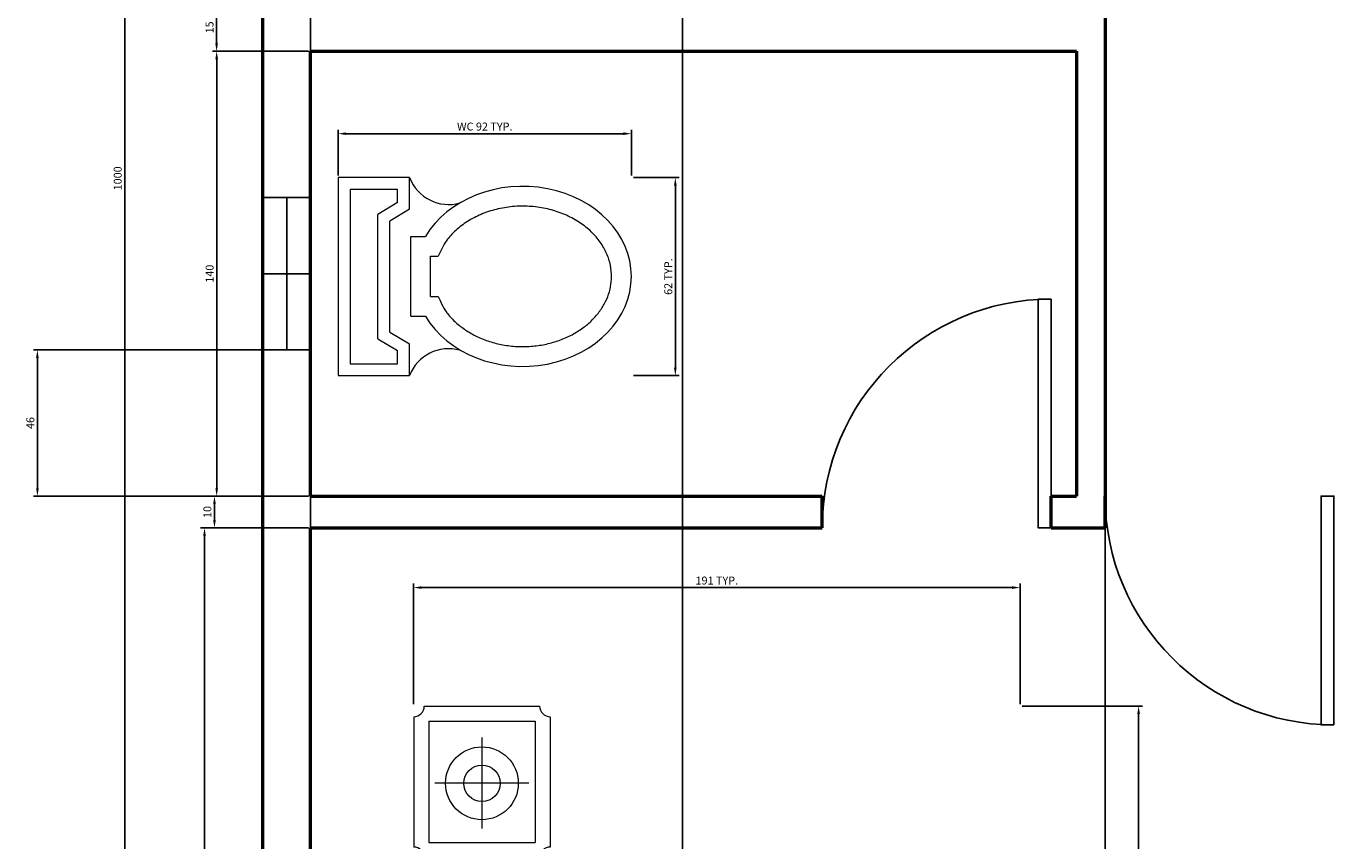
# Model space of a CAD drawing. Units: inches. Extents: x 604 to 3492, y -123 to 1737.
# Tile 12 of 20: x 1500 to 1912, y 579 to 836. Entities that reach past the tile are written whole.
import ezdxf

# ---------------------------------------------------------------- set-up
doc = ezdxf.new("R2010")
doc.units = ezdxf.units.IN
for name, color, linetype, lineweight in [('A-ANNO-DIMS', 2, 'Continuous', 18), ('A-DOOR', 3, 'Continuous', 25), ('A-FLOR-FIXT', 9, 'Continuous', 18), ('A-FURN', 8, 'Continuous', 18), ('A-GLAZ', 4, 'Continuous', 25), ('A-WALL', 7, 'Continuous', 50)]:
    doc.layers.add(name, color=color, linetype=linetype, lineweight=lineweight)
doc.styles.get("Standard").update_dxf_attribs({"font": 'arial.ttf'})
doc.dimstyles.new('ISO-25', dxfattribs={"dimtxt": 2.5, "dimasz": 2.5, "dimexe": 1.25, "dimexo": 0.625, "dimtad": 1, "dimtxsty": 'Standard', "dimcen": 2.5, "dimadec": 0, "dimazin": 0, "dimtfac": 1, "dimtmove": 0, "dimatfit": 3, "dimfxl": 1, "dimarcsym": 0})

# ---------------------------------------------------------------- blocks, each defined once
blk = doc.blocks.new('A$C7C8779AE')
for p, q in [((0, 0.7405), (0, 0.5605)), ((0.5, 0.7405), (0, 0.7405)), ((0.5, 0.5605), (0.5, 0.7405)), ((0.47, 0.7105), (0.03, 0.7105)), ((0.03, 0.7105), (0.03, 0.5905)), ((0.47, 0.5905), (0.47, 0.7105)), ((0.093, 0.6405), (0.063, 0.5905)), ((0.093, 0.6405), (0.407, 0.6405)), ((0.437, 0.5905), (0.407, 0.6405)), ((0.11, 0.6105), (0.08, 0.5605)), ((0.11, 0.6105), (0.39, 0.6105)), ((0.42, 0.5605), (0.39, 0.6105)), ((0.03, 0.5905), (0.063, 0.5905)), ((0.437, 0.5905), (0.47, 0.5905)), ((0, 0.5605), (0.08, 0.5605)), ((0.1497, 0.557), (0.1497, 0.5203)), ((0.1497, 0.557), (0.3514, 0.557)), ((0.3514, 0.557), (0.3514, 0.5203)), ((0.42, 0.5605), (0.5, 0.5605)), ((0.1997, 0.507), (0.1997, 0.4879)), ((0.1997, 0.507), (0.3014, 0.507)), ((0.3014, 0.507), (0.3014, 0.4879))]:
    blk.add_line(p, q)
for centre, start, end in [((-0.0386, 0.4613), 344.642, 68.7339), ((0.5386, 0.4613), 111.2661, 195.358)]:
    blk.add_arc(centre, 0.1064, start, end)
blk.add_ellipse((0.2506, 0.2744), major_axis=(0, 0.2744), ratio=0.828948, start_param=0.459479, end_param=5.823706)
blk.add_open_spline([(0.1997, 0.4879), (0.1697, 0.474), (0.1642, 0.4702), (0.1512, 0.4602), (0.1438, 0.4535), (0.1298, 0.4388), (0.1233, 0.4306), (0.1111, 0.4131), (0.1055, 0.4037), (0.0956, 0.3838), (0.0912, 0.3733), (0.0838, 0.3516), (0.0808, 0.3403), (0.0762, 0.3172), (0.0746, 0.3055), (0.073, 0.2817), (0.0729, 0.2698), (0.0743, 0.246), (0.0758, 0.2342), (0.0801, 0.2111), (0.0831, 0.1998), (0.0903, 0.1779), (0.0945, 0.1673), (0.1043, 0.1473), (0.1098, 0.1378), (0.1218, 0.12), (0.1283, 0.1118), (0.1421, 0.0968), (0.1494, 0.09), (0.1646, 0.078), (0.1725, 0.0728), (0.1887, 0.064), (0.1969, 0.0603), (0.2137, 0.0547), (0.2222, 0.0527), (0.2392, 0.0502), (0.2478, 0.0498), (0.2664, 0.0505), (0.2764, 0.052), (0.2963, 0.0573), (0.3061, 0.061), (0.3253, 0.0707), (0.3346, 0.0766), (0.3525, 0.0906), (0.3611, 0.0987), (0.3771, 0.1169), (0.3845, 0.127), (0.3978, 0.1488), (0.4037, 0.1605), (0.4137, 0.1853), (0.4178, 0.1983), (0.424, 0.2251), (0.4261, 0.2389), (0.4282, 0.2668), (0.4283, 0.2809), (0.4262, 0.3088), (0.4241, 0.3226), (0.418, 0.3495), (0.414, 0.3625), (0.404, 0.3873), (0.3982, 0.3991), (0.385, 0.421), (0.3776, 0.4311), (0.3617, 0.4494), (0.3531, 0.4575), (0.3382, 0.4693), (0.3321, 0.4736), (0.3014, 0.4879)], degree=3, knots=[0.459479, 0.459479, 0.459479, 0.459479, 0.567422, 0.567422, 0.720865, 0.720865, 0.874307, 0.874307, 1.02775, 1.02775, 1.181192, 1.181192, 1.334635, 1.334635, 1.488077, 1.488077, 1.64152, 1.64152, 1.794963, 1.794963, 1.948405, 1.948405, 2.101848, 2.101848, 2.25529, 2.25529, 2.408733, 2.408733, 2.562175, 2.562175, 2.715618, 2.715618, 2.86906, 2.86906, 3.022503, 3.022503, 3.175946, 3.175946, 3.356457, 3.356457, 3.536968, 3.536968, 3.717479, 3.717479, 3.89799, 3.89799, 4.078501, 4.078501, 4.259012, 4.259012, 4.439523, 4.439523, 4.620035, 4.620035, 4.800546, 4.800546, 4.981057, 4.981057, 5.161568, 5.161568, 5.342079, 5.342079, 5.52259, 5.52259, 5.703101, 5.703101, 5.823706, 5.823706, 5.823706, 5.823706])
blk = doc.blocks.new('A$C50B66110')
for p, q in [((0.0503, 1.9981), (0.4803, 1.9981)), ((0.1513, 1.6871), (0.1513, 1.9967)), ((0.5716, 1.9488), (0.5716, 2)), ((0.5716, 2), (2.0719, 2)), ((2.0719, 1.9488), (2.0719, 2)), ((2.5701, 1.9993), (2.1401, 1.9993)), ((0.0153, 1.9631), (0.0153, 1.5831)), ((0.0653, 1.9481), (0.0653, 1.5981)), ((0.0653, 1.9481), (0.4653, 1.9481)), ((0.4653, 1.9481), (0.4653, 1.5981)), ((0.5153, 1.9631), (0.5153, 1.5831)), ((2.0719, 1.9488), (0.5716, 1.9488)), ((0.5716, 1.9488), (0.5716, 0)), ((2.0719, 0), (2.0719, 1.9488)), ((2.1051, 1.9643), (2.1051, 1.5843)), ((2.1551, 1.9493), (2.1551, 1.5993)), ((2.5551, 1.9493), (2.1551, 1.9493)), ((2.5551, 1.9493), (2.5551, 1.5993)), ((2.6051, 1.9643), (2.6051, 1.5843)), ((2.3505, 1.62), (2.3505, 1.9295)), ((0.7257, 1.5725), (0.7257, 1.8954)), ((0.7257, 1.8954), (1.2113, 1.8954)), ((1.2113, 1.8954), (1.2113, 1.5725)), ((1.4007, 1.5725), (1.4007, 1.8954)), ((1.4007, 1.8954), (1.8863, 1.8954)), ((1.8863, 1.8954), (1.8863, 1.5725)), ((0, 1.8416), (0.2001, 1.8416)), ((2.5018, 1.7744), (2.2017, 1.7744)), ((0.0653, 1.5981), (0.4653, 1.5981)), ((2.5551, 1.5993), (2.1551, 1.5993)), ((1.2113, 1.5725), (0.7257, 1.5725)), ((1.8863, 1.5725), (1.4007, 1.5725)), ((0.0503, 1.5481), (0.4803, 1.5481)), ((1.5665, 1.5254), (1.5665, 1.0802)), ((1.5665, 1.5254), (1.9219, 1.0802)), ((2.5701, 1.5493), (2.1401, 1.5493)), ((1.9219, 1.0802), (1.5665, 1.0802)), ((0.5716, 0), (0.7216, 0.15)), ((2.0719, 0), (1.9219, 0.15)), ((0.5716, 0), (2.0719, 0))]:
    blk.add_line(p, q)
at = {"linetype": 'ByBlock'}
for p, q in [((0.2481, 1.9162), (0.2458, 1.9139)), ((0.2458, 1.9139), (0.2458, 1.7562)), ((0.2481, 1.9162), (0.4287, 1.9162)), ((0.2526, 1.9036), (0.2526, 1.8431)), ((0.3669, 1.9036), (0.2526, 1.9036)), ((0.3669, 1.8431), (0.3669, 1.9036)), ((0.3772, 1.9071), (0.3818, 1.9128)), ((0.3772, 1.7688), (0.3772, 1.9071)), ((0.3818, 1.9094), (0.3807, 1.9048)), ((0.3807, 1.9048), (0.3807, 1.8739)), ((0.3807, 1.9048), (0.3909, 1.8945)), ((0.3818, 1.9128), (0.4161, 1.9128)), ((0.3864, 1.9116), (0.3818, 1.9094)), ((0.3921, 1.8968), (0.3864, 1.9116)), ((0.3864, 1.9116), (0.4138, 1.9116)), ((0.4081, 1.8968), (0.4138, 1.9116)), ((0.4195, 1.9048), (0.4092, 1.8945)), ((0.4138, 1.9116), (0.4184, 1.9094)), ((0.4161, 1.9128), (0.4218, 1.9071)), ((0.4184, 1.9094), (0.4195, 1.9048)), ((0.4195, 1.9048), (0.4195, 1.8739)), ((0.4218, 1.9071), (0.4218, 1.7699)), ((0.4287, 1.9162), (0.4309, 1.9139)), ((0.4309, 1.9139), (0.4309, 1.7562)), ((0.3807, 1.8739), (0.3829, 1.8682)), ((0.3829, 1.8682), (0.3864, 1.8625)), ((0.3864, 1.8625), (0.3875, 1.8545)), ((0.3875, 1.8545), (0.3875, 1.8431)), ((0.3909, 1.8945), (0.3921, 1.8968)), ((0.3909, 1.8431), (0.3909, 1.8945)), ((0.4081, 1.8968), (0.3921, 1.8968)), ((0.4092, 1.8945), (0.4081, 1.8968)), ((0.4092, 1.8431), (0.4092, 1.8945)), ((0.4138, 1.8625), (0.4127, 1.8545)), ((0.4127, 1.8545), (0.4127, 1.8431)), ((0.4172, 1.8682), (0.4138, 1.8625)), ((0.4195, 1.8739), (0.4172, 1.8682)), ((0.2526, 1.8431), (0.3669, 1.8431)), ((0.3201, 1.8168), (0.2526, 1.8168)), ((0.2526, 1.8168), (0.2526, 1.7962)), ((0.2572, 1.8408), (0.2572, 1.8294)), ((0.3669, 1.8408), (0.2572, 1.8408)), ((0.2572, 1.8294), (0.3669, 1.8294)), ((0.2675, 1.8145), (0.2641, 1.8145)), ((0.2641, 1.8145), (0.2641, 1.8111)), ((0.2641, 1.8111), (0.2675, 1.8111)), ((0.2664, 1.8408), (0.2664, 1.8294)), ((0.2675, 1.8111), (0.2675, 1.8145)), ((0.2755, 1.8408), (0.2755, 1.8294)), ((0.2846, 1.8408), (0.2846, 1.8294)), ((0.2846, 1.8145), (0.2846, 1.8111)), ((0.2881, 1.8145), (0.2846, 1.8145)), ((0.2846, 1.8111), (0.2881, 1.8111)), ((0.2881, 1.8111), (0.2881, 1.8145)), ((0.2938, 1.8408), (0.2938, 1.8294)), ((0.3029, 1.8408), (0.3029, 1.8294)), ((0.3052, 1.8145), (0.3052, 1.8111)), ((0.3086, 1.8145), (0.3052, 1.8145)), ((0.3052, 1.8111), (0.3086, 1.8111)), ((0.3086, 1.8111), (0.3086, 1.8145)), ((0.3121, 1.8408), (0.3121, 1.8294)), ((0.3201, 1.7962), (0.3201, 1.8168)), ((0.3304, 1.8111), (0.3395, 1.8111)), ((0.3304, 1.8042), (0.3304, 1.8111)), ((0.3395, 1.8111), (0.3395, 1.8042)), ((0.3441, 1.8042), (0.3441, 1.8111)), ((0.3441, 1.8111), (0.3532, 1.8111)), ((0.3532, 1.8111), (0.3532, 1.8042)), ((0.3578, 1.8111), (0.3669, 1.8111)), ((0.3578, 1.8042), (0.3578, 1.8111)), ((0.3669, 1.8294), (0.3669, 1.8408)), ((0.3669, 1.8111), (0.3669, 1.8042)), ((0.3829, 1.8076), (0.3864, 1.8134)), ((0.3864, 1.8134), (0.3875, 1.8214)), ((0.3875, 1.8214), (0.3875, 1.8431)), ((0.3909, 1.8431), (0.3909, 1.7813)), ((0.4092, 1.8431), (0.4092, 1.7813)), ((0.4127, 1.8214), (0.4127, 1.8431)), ((0.4138, 1.8134), (0.4127, 1.8214)), ((0.4172, 1.8076), (0.4138, 1.8134)), ((0.2526, 1.7962), (0.3201, 1.7962)), ((0.2652, 1.7905), (0.2538, 1.7905)), ((0.2538, 1.7905), (0.2538, 1.7859)), ((0.2538, 1.7859), (0.2652, 1.7859)), ((0.2538, 1.7665), (0.2538, 1.7733)), ((0.2538, 1.7733), (0.2652, 1.7733)), ((0.2641, 1.8019), (0.2641, 1.7985)), ((0.2675, 1.8019), (0.2641, 1.8019)), ((0.2641, 1.7985), (0.2675, 1.7985)), ((0.2652, 1.7859), (0.2652, 1.7905)), ((0.2652, 1.7733), (0.2652, 1.7665)), ((0.2675, 1.7985), (0.2675, 1.8019)), ((0.2812, 1.7905), (0.2698, 1.7905)), ((0.2698, 1.7905), (0.2698, 1.7859)), ((0.2698, 1.7859), (0.2812, 1.7859)), ((0.2698, 1.7665), (0.2698, 1.7733)), ((0.2698, 1.7733), (0.2812, 1.7733)), ((0.2812, 1.7859), (0.2812, 1.7905)), ((0.2812, 1.7733), (0.2812, 1.7665)), ((0.2846, 1.8019), (0.2846, 1.7985)), ((0.2881, 1.8019), (0.2846, 1.8019)), ((0.2846, 1.7985), (0.2881, 1.7985)), ((0.2972, 1.7905), (0.2858, 1.7905)), ((0.2858, 1.7905), (0.2858, 1.7859)), ((0.2858, 1.7859), (0.2972, 1.7859)), ((0.2858, 1.7665), (0.2858, 1.7733)), ((0.2858, 1.7733), (0.2972, 1.7733)), ((0.2881, 1.7985), (0.2881, 1.8019)), ((0.2972, 1.7859), (0.2972, 1.7905)), ((0.2972, 1.7733), (0.2972, 1.7665)), ((0.3018, 1.7905), (0.3018, 1.7859)), ((0.3132, 1.7905), (0.3018, 1.7905)), ((0.3018, 1.7859), (0.3132, 1.7859)), ((0.3018, 1.7733), (0.3132, 1.7733)), ((0.3018, 1.7665), (0.3018, 1.7733)), ((0.3052, 1.8019), (0.3052, 1.7985)), ((0.3086, 1.8019), (0.3052, 1.8019)), ((0.3052, 1.7985), (0.3086, 1.7985)), ((0.3086, 1.7985), (0.3086, 1.8019)), ((0.3132, 1.7859), (0.3132, 1.7905)), ((0.3132, 1.7733), (0.3132, 1.7665)), ((0.3395, 1.8042), (0.3304, 1.8042)), ((0.3304, 1.7985), (0.3395, 1.7985)), ((0.3304, 1.7916), (0.3304, 1.7985)), ((0.3395, 1.7916), (0.3304, 1.7916)), ((0.3304, 1.7779), (0.3304, 1.7848)), ((0.3304, 1.7848), (0.3395, 1.7848)), ((0.3395, 1.7779), (0.3304, 1.7779)), ((0.3304, 1.7722), (0.3395, 1.7722)), ((0.3304, 1.7653), (0.3304, 1.7722)), ((0.3395, 1.7985), (0.3395, 1.7916)), ((0.3395, 1.7848), (0.3395, 1.7779)), ((0.3395, 1.7722), (0.3395, 1.7653)), ((0.3532, 1.8042), (0.3441, 1.8042)), ((0.3441, 1.7985), (0.3532, 1.7985)), ((0.3441, 1.7916), (0.3441, 1.7985)), ((0.3532, 1.7916), (0.3441, 1.7916)), ((0.3441, 1.7779), (0.3441, 1.7848)), ((0.3441, 1.7848), (0.3532, 1.7848)), ((0.3532, 1.7779), (0.3441, 1.7779)), ((0.3441, 1.7722), (0.3532, 1.7722)), ((0.3441, 1.7653), (0.3441, 1.7722)), ((0.3532, 1.7985), (0.3532, 1.7916)), ((0.3532, 1.7848), (0.3532, 1.7779)), ((0.3532, 1.7722), (0.3532, 1.7653)), ((0.3669, 1.8042), (0.3578, 1.8042)), ((0.3578, 1.7985), (0.3669, 1.7985)), ((0.3578, 1.7916), (0.3578, 1.7985)), ((0.3669, 1.7916), (0.3578, 1.7916)), ((0.3578, 1.7791), (0.3578, 1.7859)), ((0.3578, 1.7859), (0.3669, 1.7859)), ((0.3669, 1.7791), (0.3578, 1.7791)), ((0.3578, 1.7653), (0.3578, 1.7722)), ((0.3578, 1.7722), (0.3669, 1.7722)), ((0.3669, 1.7985), (0.3669, 1.7916)), ((0.3669, 1.7859), (0.3669, 1.7791)), ((0.3669, 1.7722), (0.3669, 1.7653)), ((0.3829, 1.7631), (0.3772, 1.7688)), ((0.3807, 1.8019), (0.3829, 1.8076)), ((0.3807, 1.7711), (0.3807, 1.8019)), ((0.3807, 1.7711), (0.3909, 1.7813)), ((0.3818, 1.7665), (0.3807, 1.7711)), ((0.3921, 1.7791), (0.3864, 1.7642)), ((0.3909, 1.7813), (0.3921, 1.7791)), ((0.4081, 1.7791), (0.3921, 1.7791)), ((0.4092, 1.7813), (0.4081, 1.7791)), ((0.4081, 1.7791), (0.4138, 1.7642)), ((0.4195, 1.7711), (0.4092, 1.7813)), ((0.4218, 1.7699), (0.4161, 1.7631)), ((0.4195, 1.8019), (0.4172, 1.8076)), ((0.4184, 1.7665), (0.4195, 1.7711)), ((0.4195, 1.7711), (0.4195, 1.8019)), ((0.4378, 1.7742), (0.4309, 1.7768)), ((0.4309, 1.7722), (0.436, 1.7708)), ((0.436, 1.7708), (0.4406, 1.7672)), ((0.441, 1.771), (0.4378, 1.7742)), ((0.4434, 1.7688), (0.441, 1.771)), ((0.4477, 1.7704), (0.4434, 1.7688)), ((0.4497, 1.7684), (0.4477, 1.7704)), ((0.4481, 1.765), (0.4497, 1.7684)), ((0.2458, 1.7562), (0.2481, 1.7539)), ((0.4, 1.7539), (0.2481, 1.7539)), ((0.2652, 1.7665), (0.2538, 1.7665)), ((0.2812, 1.7665), (0.2698, 1.7665)), ((0.2972, 1.7665), (0.2858, 1.7665)), ((0.3132, 1.7665), (0.3018, 1.7665)), ((0.3395, 1.7653), (0.3304, 1.7653)), ((0.3532, 1.7653), (0.3441, 1.7653)), ((0.3669, 1.7653), (0.3578, 1.7653)), ((0.3864, 1.7642), (0.3818, 1.7665)), ((0.399, 1.7631), (0.3829, 1.7631)), ((0.3864, 1.7642), (0.399, 1.7642)), ((0.4024, 1.7676), (0.3989, 1.7676)), ((0.3989, 1.7676), (0.3991, 1.7578)), ((0.3991, 1.7578), (0.4019, 1.7462)), ((0.4019, 1.7462), (0.4047, 1.7353)), ((0.4026, 1.7254), (0.4021, 1.7198)), ((0.403, 1.7585), (0.4024, 1.7676)), ((0.4026, 1.7642), (0.4138, 1.7642)), ((0.4051, 1.7279), (0.4026, 1.7254)), ((0.4161, 1.7631), (0.4027, 1.7631)), ((0.4047, 1.7511), (0.403, 1.7585)), ((0.4287, 1.7539), (0.404, 1.7539)), ((0.4047, 1.7353), (0.4044, 1.7293)), ((0.4044, 1.7293), (0.4051, 1.7279)), ((0.4074, 1.7402), (0.4047, 1.7511)), ((0.4081, 1.7346), (0.4074, 1.7402)), ((0.4079, 1.7286), (0.4081, 1.7346)), ((0.4121, 1.7256), (0.4079, 1.7286)), ((0.4111, 1.7203), (0.4121, 1.7256)), ((0.4138, 1.7642), (0.4184, 1.7665)), ((0.4309, 1.7562), (0.4287, 1.7539)), ((0.4406, 1.7672), (0.4418, 1.7656)), ((0.4443, 1.7658), (0.4418, 1.7633)), ((0.4418, 1.7656), (0.4443, 1.7658)), ((0.4418, 1.7633), (0.4511, 1.7551)), ((0.4509, 1.7672), (0.4481, 1.765)), ((0.4539, 1.764), (0.4509, 1.7672)), ((0.4511, 1.7551), (0.4662, 1.7422)), ((0.4515, 1.7573), (0.4539, 1.764)), ((0.4577, 1.7605), (0.4515, 1.7573)), ((0.463, 1.7555), (0.4577, 1.7605)), ((0.4618, 1.7482), (0.463, 1.7555)), ((0.467, 1.7515), (0.4618, 1.7482)), ((0.4664, 1.7418), (0.4741, 1.72)), ((0.4714, 1.7468), (0.467, 1.7515)), ((0.4696, 1.7418), (0.4714, 1.7468)), ((0.4766, 1.7425), (0.4697, 1.7418)), ((0.472, 1.733), (0.4787, 1.7356)), ((0.4794, 1.7332), (0.472, 1.733)), ((0.4761, 1.7233), (0.481, 1.7279)), ((0.4787, 1.7356), (0.4766, 1.7425)), ((0.481, 1.7279), (0.4794, 1.7332)), ((0.4021, 1.7198), (0.4088, 1.7187)), ((0.4088, 1.7187), (0.4023, 1.7147)), ((0.4023, 1.7147), (0.4028, 1.7085)), ((0.4028, 1.7085), (0.4102, 1.7078)), ((0.4102, 1.7078), (0.4037, 1.7027)), ((0.4037, 1.7027), (0.4067, 1.6974)), ((0.4067, 1.6974), (0.4137, 1.6988)), ((0.4137, 1.6988), (0.4104, 1.6923)), ((0.4104, 1.6923), (0.4139, 1.6881)), ((0.4123, 1.7057), (0.4111, 1.7203)), ((0.4211, 1.6946), (0.4123, 1.7057)), ((0.4139, 1.6881), (0.4192, 1.692)), ((0.4192, 1.692), (0.4183, 1.6858)), ((0.4183, 1.6858), (0.4227, 1.683)), ((0.4333, 1.6881), (0.4211, 1.6946)), ((0.4227, 1.683), (0.4283, 1.6876)), ((0.4283, 1.6876), (0.4276, 1.68)), ((0.4324, 1.6786), (0.4354, 1.6849)), ((0.4472, 1.6869), (0.4333, 1.6881)), ((0.4354, 1.6849), (0.4382, 1.6786)), ((0.4421, 1.6782), (0.4437, 1.6849)), ((0.4437, 1.6849), (0.4463, 1.6775)), ((0.4606, 1.6927), (0.4472, 1.6869)), ((0.4507, 1.6786), (0.4509, 1.6849)), ((0.4509, 1.6849), (0.4562, 1.6802)), ((0.4562, 1.6802), (0.4599, 1.6821)), ((0.4592, 1.689), (0.4641, 1.683)), ((0.4599, 1.6821), (0.4592, 1.689)), ((0.4708, 1.7027), (0.4606, 1.6927)), ((0.4641, 1.683), (0.4678, 1.6863)), ((0.465, 1.6925), (0.4715, 1.6897)), ((0.4678, 1.6863), (0.465, 1.6925)), ((0.4741, 1.72), (0.4708, 1.7027)), ((0.4745, 1.6925), (0.4713, 1.6988)), ((0.4713, 1.6988), (0.478, 1.6967)), ((0.4715, 1.6897), (0.4745, 1.6925)), ((0.4743, 1.7075), (0.4815, 1.7073)), ((0.4798, 1.7013), (0.4743, 1.7075)), ((0.4824, 1.7233), (0.4761, 1.7233)), ((0.4764, 1.7154), (0.4835, 1.7175)), ((0.4824, 1.7119), (0.4764, 1.7154)), ((0.478, 1.6967), (0.4798, 1.7013)), ((0.4815, 1.7073), (0.4824, 1.7119)), ((0.4835, 1.7175), (0.4824, 1.7233)), ((0.4276, 1.68), (0.4324, 1.6786)), ((0.4382, 1.6786), (0.4421, 1.6782)), ((0.4463, 1.6775), (0.4507, 1.6786)), ((0.7216, 1.5254), (1.9219, 1.5254)), ((0.7216, 1.5254), (0.7216, 0.15)), ((1.9219, 0.15), (1.9219, 1.5254)), ((0.7216, 0.15), (1.9219, 0.15))]:
    blk.add_line(p, q, dxfattribs=at)
for centre, radius in [((0.1513, 1.8416), 0.12), ((0.1513, 1.8416), 0.06), ((2.3505, 1.7744), 0.12), ((2.3505, 1.7744), 0.06)]:
    blk.add_circle(centre, radius)
for centre, radius, start, end in [((0.0153, 1.9981), 0.035, 270, 0), ((0.5153, 1.9981), 0.035, 180, 270), ((2.1051, 1.9993), 0.035, 270, 0), ((2.6051, 1.9993), 0.035, 180, 270), ((0.6244, 1.734), 0.1906, 302.1202, 57.8798), ((1.3126, 1.734), 0.1906, 122.1202, 237.8798), ((1.2994, 1.734), 0.1906, 302.1202, 57.8798), ((1.9876, 1.734), 0.1906, 122.1202, 237.8798), ((0.0153, 1.5481), 0.035, 0, 90), ((0.5153, 1.5481), 0.035, 90, 180), ((2.1051, 1.5493), 0.035, 0, 90), ((2.6051, 1.5493), 0.035, 90, 180), ((1.1502, 0.7366), 0.3575, 102.4782, 140.4625), ((0.328, 0.4368), 0.9879, 28.4971, 41.0566), ((1.9117, 1.3157), 0.8697, 195.336, 226.4193), ((0.9996, 0.4307), 0.548, 103.2034, 117.0362), ((1.656, 1.7093), 1.0798, 223.6306, 251.4288), ((0.4482, 0.4408), 0.5655, 5.3391, 57.6895), ((1.8226, 1.3753), 1.1652, 203.0642, 220.3209), ((0.4548, 0.5307), 0.4879, 10.6986, 52.6864), ((0.5648, 0.4378), 0.7874, 18.3527, 36.6851), ((1.4166, 0.4903), 0.3575, 154.0418, 192.0262), ((1.1403, -0.3401), 0.9879, 80.0607, 92.6202), ((-0.0179, 2.4352), 2.1977, 305.2966, 307.2418), ((1.5981, 0.9345), 0.734, 205.259, 216.9351), ((1.3672, 0.0075), 0.6085, 71.81, 120.1351), ((1.2867, -0.154), 0.7874, 69.9163, 88.2487), ((1.4431, 0.1219), 0.4774, 76.1849, 142.0017), ((-0.6401, 0.6314), 2.1977, 349.4884, 358.8054), ((-0.0179, 2.4352), 2.1977, 297.9248, 299.3793), ((1.5626, 0.1822), 0.548, 154.767, 168.5998), ((1.2678, 0.9611), 0.6885, 250.2936, 293.6414), ((1.3343, 1.4141), 1.1652, 254.6278, 271.8845), ((1.5399, 0.9642), 0.734, 256.8226, 268.4988)]:
    blk.add_arc(centre, radius, start, end)
blk = doc.blocks.new('*D64')
at = {"layer": 'A-ANNO-DIMS', "color": 0, "lineweight": -2, "transparency": 16777216}
for p, q in [((1588.95, 842.7), (1558.76, 842.7)), ((1560.01, 840.2), (1560.01, 830.2)), ((1588.95, 827.7), (1558.76, 827.7))]:
    blk.add_line(p, q, dxfattribs=at)
at = {"layer": 'A-ANNO-DIMS', "color": 0, "transparency": 16777216}
for points in [[(1559.6, 840.2), (1560.43, 840.2), (1560.01, 842.7)], [(1559.6, 830.2), (1560.43, 830.2), (1560.01, 827.7)]]:
    blk.add_solid(points, dxfattribs=at)
at = {"layer": 'Defpoints', "color": 0, "transparency": 16777216}
for p in [(1589.57, 842.7), (1560.01, 827.7), (1589.57, 827.7)]:
    blk.add_point(p, dxfattribs=at)
at = {"layer": 'A-ANNO-DIMS', "color": 0, "transparency": 16777216, "insert": (1558.11, 835.2), "char_height": 2.5, "attachment_point": 5, "rotation": 90}
blk.add_mtext('15', dxfattribs=at)
blk = doc.blocks.new('*D65')
at = {"layer": 'A-ANNO-DIMS', "color": 0, "lineweight": -2, "transparency": 16777216}
for p, q in [((1588.95, 827.7), (1558.79, 827.7)), ((1560.04, 825.2), (1560.04, 690.2)), ((1588.95, 687.7), (1558.79, 687.7))]:
    blk.add_line(p, q, dxfattribs=at)
at = {"layer": 'A-ANNO-DIMS', "color": 0, "transparency": 16777216}
for points in [[(1559.62, 825.2), (1560.46, 825.2), (1560.04, 827.7)], [(1559.62, 690.2), (1560.46, 690.2), (1560.04, 687.7)]]:
    blk.add_solid(points, dxfattribs=at)
at = {"layer": 'Defpoints', "color": 0, "transparency": 16777216}
for p in [(1589.57, 827.7), (1560.04, 687.7), (1589.57, 687.7)]:
    blk.add_point(p, dxfattribs=at)
at = {"layer": 'A-ANNO-DIMS', "color": 0, "transparency": 16777216, "insert": (1558.14, 757.7), "char_height": 2.5, "attachment_point": 5, "rotation": 90}
blk.add_mtext('140', dxfattribs=at)
blk = doc.blocks.new('*D66')
at = {"layer": 'A-ANNO-DIMS', "color": 0, "lineweight": -2, "transparency": 16777216}
for p, q in [((1588.95, 687.7), (1558.09, 687.7)), ((1559.34, 685.2), (1559.34, 680.2)), ((1588.95, 677.7), (1558.09, 677.7))]:
    blk.add_line(p, q, dxfattribs=at)
at = {"layer": 'A-ANNO-DIMS', "color": 0, "transparency": 16777216}
for points in [[(1558.92, 685.2), (1559.76, 685.2), (1559.34, 687.7)], [(1558.92, 680.2), (1559.76, 680.2), (1559.34, 677.7)]]:
    blk.add_solid(points, dxfattribs=at)
at = {"layer": 'Defpoints', "color": 0, "transparency": 16777216}
for p in [(1589.57, 687.7), (1559.34, 677.7), (1589.57, 677.7)]:
    blk.add_point(p, dxfattribs=at)
at = {"layer": 'A-ANNO-DIMS', "color": 0, "transparency": 16777216, "insert": (1557.44, 682.7), "char_height": 2.5, "attachment_point": 5, "rotation": 90}
blk.add_mtext('10', dxfattribs=at)
blk = doc.blocks.new('*D67')
at = {"layer": 'A-ANNO-DIMS', "color": 0, "lineweight": -2, "transparency": 16777216}
for p, q in [((1588.95, 677.7), (1554.96, 677.7)), ((1556.21, 675.2), (1556.21, 305.2)), ((1588.95, 302.7), (1554.96, 302.7))]:
    blk.add_line(p, q, dxfattribs=at)
at = {"layer": 'A-ANNO-DIMS', "color": 0, "transparency": 16777216}
for points in [[(1555.79, 675.2), (1556.62, 675.2), (1556.21, 677.7)], [(1555.79, 305.2), (1556.62, 305.2), (1556.21, 302.7)]]:
    blk.add_solid(points, dxfattribs=at)
at = {"layer": 'Defpoints', "color": 0, "transparency": 16777216}
for p in [(1589.57, 677.7), (1556.21, 302.7), (1589.57, 302.7)]:
    blk.add_point(p, dxfattribs=at)
at = {"layer": 'A-ANNO-DIMS', "color": 0, "transparency": 16777216, "insert": (1554.3, 490.2), "char_height": 2.5, "attachment_point": 5, "rotation": 90}
blk.add_mtext('375', dxfattribs=at)
blk = doc.blocks.new('*D69')
at = {"layer": 'A-ANNO-DIMS', "color": 0, "lineweight": -2, "transparency": 16777216}
for p, q in [((1573.95, 1287.7), (1529.86, 1287.7)), ((1531.11, 290.2), (1531.11, 1285.2)), ((1573.95, 287.7), (1529.86, 287.7))]:
    blk.add_line(p, q, dxfattribs=at)
at = {"layer": 'A-ANNO-DIMS', "color": 0, "transparency": 16777216}
for points in [[(1530.69, 1285.2), (1531.52, 1285.2), (1531.11, 1287.7)], [(1530.69, 290.2), (1531.52, 290.2), (1531.11, 287.7)]]:
    blk.add_solid(points, dxfattribs=at)
at = {"layer": 'Defpoints', "color": 0, "transparency": 16777216}
for p in [(1531.11, 1287.7), (1574.57, 1287.7), (1574.57, 287.7)]:
    blk.add_point(p, dxfattribs=at)
at = {"layer": 'A-ANNO-DIMS', "color": 0, "transparency": 16777216, "insert": (1529.21, 787.7), "char_height": 2.5, "attachment_point": 5, "rotation": 90}
blk.add_mtext('1000', dxfattribs=at)
blk = doc.blocks.new('DOOR-SWING-72')
for p, q in [((0, 72), (0, 0)), ((0, 0), (4, 0)), ((0, 0), (4, 0))]:
    blk.add_line(p, q)
blk.add_lwpolyline([(0, 72), (0, 0), (4, 0), (4, 72)], close=True)
blk.add_arc((0, 0), 72, 0, 90)
blk = doc.blocks.new('WIN-48')
for p, q in [((0, 48), (15, 48)), ((7.5, 48), (7.5, 0)), ((15, 48), (15, 0)), ((0, 24), (15, 24))]:
    blk.add_line(p, q)
blk.add_lwpolyline([(15, 0), (0, 0), (0, 48), (15, 48)], close=True)
blk = doc.blocks.new('*D75')
at = {"layer": 'A-ANNO-DIMS', "color": 0, "lineweight": -2, "transparency": 16777216}
for p, q in [((1598.28, 788.55), (1598.28, 803.01)), ((1690.52, 788.55), (1690.52, 803.01)), ((1688.02, 801.76), (1600.78, 801.76))]:
    blk.add_line(p, q, dxfattribs=at)
at = {"layer": 'A-ANNO-DIMS', "color": 0, "transparency": 16777216}
for points in [[(1600.78, 802.18), (1600.78, 801.35), (1598.28, 801.76)], [(1688.02, 802.18), (1688.02, 801.35), (1690.52, 801.76)]]:
    blk.add_solid(points, dxfattribs=at)
at = {"layer": 'Defpoints', "color": 0, "transparency": 16777216}
for p in [(1598.28, 801.76), (1598.28, 787.93), (1690.52, 787.93)]:
    blk.add_point(p, dxfattribs=at)
at = {"layer": 'A-ANNO-DIMS', "color": 0, "transparency": 16777216, "insert": (1644.4, 803.68), "char_height": 2.5, "attachment_point": 5}
blk.add_mtext('WC 92 TYP.', dxfattribs=at)
blk = doc.blocks.new('*D76')
at = {"layer": 'A-ANNO-DIMS', "color": 0, "lineweight": -2, "transparency": 16777216}
for p, q in [((1691.15, 787.93), (1705.61, 787.93)), ((1704.36, 728.14), (1704.36, 785.43)), ((1691.15, 725.64), (1705.61, 725.64))]:
    blk.add_line(p, q, dxfattribs=at)
at = {"layer": 'A-ANNO-DIMS', "color": 0, "transparency": 16777216}
for points in [[(1703.94, 785.43), (1704.77, 785.43), (1704.36, 787.93)], [(1703.94, 728.14), (1704.77, 728.14), (1704.36, 725.64)]]:
    blk.add_solid(points, dxfattribs=at)
at = {"layer": 'Defpoints', "color": 0, "transparency": 16777216}
for p in [(1690.52, 787.93), (1704.36, 787.93), (1690.52, 725.64)]:
    blk.add_point(p, dxfattribs=at)
at = {"layer": 'A-ANNO-DIMS', "color": 0, "transparency": 16777216, "insert": (1702.46, 756.78), "char_height": 2.5, "attachment_point": 5, "rotation": 90}
blk.add_mtext('62 TYP.', dxfattribs=at)
blk = doc.blocks.new('*D77')
at = {"layer": 'A-ANNO-DIMS', "color": 0, "lineweight": -2, "transparency": 16777216}
for p, q in [((1813.47, 621.62), (1851.39, 621.62)), ((1850.14, 375.49), (1850.14, 619.12)), ((1813.47, 372.99), (1851.39, 372.99))]:
    blk.add_line(p, q, dxfattribs=at)
at = {"layer": 'A-ANNO-DIMS', "color": 0, "transparency": 16777216}
for points in [[(1849.72, 619.12), (1850.56, 619.12), (1850.14, 621.62)], [(1849.72, 375.49), (1850.56, 375.49), (1850.14, 372.99)]]:
    blk.add_solid(points, dxfattribs=at)
at = {"layer": 'Defpoints', "color": 0, "transparency": 16777216}
for p in [(1812.84, 621.62), (1850.14, 621.62), (1812.84, 372.99)]:
    blk.add_point(p, dxfattribs=at)
at = {"layer": 'A-ANNO-DIMS', "color": 0, "transparency": 16777216, "insert": (1848.22, 497.3), "char_height": 2.5, "attachment_point": 5, "rotation": 90}
blk.add_mtext('BED SET 249 TYP.', dxfattribs=at)
blk = doc.blocks.new('*D78')
at = {"layer": 'A-ANNO-DIMS', "color": 0, "lineweight": -2, "transparency": 16777216}
for p, q in [((1621.97, 622.24), (1621.97, 660.16)), ((1810.34, 658.91), (1624.47, 658.91)), ((1812.84, 622.24), (1812.84, 660.16))]:
    blk.add_line(p, q, dxfattribs=at)
at = {"layer": 'A-ANNO-DIMS', "color": 0, "transparency": 16777216}
for points in [[(1624.47, 659.33), (1624.47, 658.5), (1621.97, 658.91)], [(1810.34, 659.33), (1810.34, 658.5), (1812.84, 658.91)]]:
    blk.add_solid(points, dxfattribs=at)
at = {"layer": 'Defpoints', "color": 0, "transparency": 16777216}
for p in [(1621.97, 658.91), (1621.97, 621.62), (1812.84, 621.62)]:
    blk.add_point(p, dxfattribs=at)
at = {"layer": 'A-ANNO-DIMS', "color": 0, "transparency": 16777216, "insert": (1717.41, 660.81), "char_height": 2.5, "attachment_point": 5}
blk.add_mtext('191 TYP.', dxfattribs=at)
blk = doc.blocks.new('*D102')
at = {"layer": 'A-ANNO-DIMS', "color": 0, "lineweight": -2, "transparency": 16777216}
for p, q in [((1839.57, 972.08), (1839.57, 215.5)), ((2023.07, 972.08), (2023.07, 215.5)), ((1842.07, 216.75), (2020.57, 216.75))]:
    blk.add_line(p, q, dxfattribs=at)
at = {"layer": 'A-ANNO-DIMS', "color": 0, "transparency": 16777216}
for points in [[(1842.07, 217.17), (1842.07, 216.33), (1839.57, 216.75)], [(2020.57, 217.17), (2020.57, 216.33), (2023.07, 216.75)]]:
    blk.add_solid(points, dxfattribs=at)
at = {"layer": 'Defpoints', "color": 0, "transparency": 16777216}
for p in [(1839.57, 972.7), (2023.07, 972.7), (2023.07, 216.75)]:
    blk.add_point(p, dxfattribs=at)
at = {"layer": 'A-ANNO-DIMS', "color": 0, "transparency": 16777216, "insert": (1931.32, 218.65), "char_height": 2.5, "attachment_point": 5}
blk.add_mtext('183.5', dxfattribs=at)
blk = doc.blocks.new('*D103')
at = {"layer": 'A-ANNO-DIMS', "color": 0, "lineweight": -2, "transparency": 16777216}
for p, q in [((1589.57, 1272.08), (1589.57, 215.5)), ((1706.57, 1272.08), (1706.57, 215.5)), ((1592.07, 216.75), (1704.07, 216.75))]:
    blk.add_line(p, q, dxfattribs=at)
at = {"layer": 'A-ANNO-DIMS', "color": 0, "transparency": 16777216}
for points in [[(1592.07, 217.17), (1592.07, 216.33), (1589.57, 216.75)], [(1704.07, 217.17), (1704.07, 216.33), (1706.57, 216.75)]]:
    blk.add_solid(points, dxfattribs=at)
at = {"layer": 'Defpoints', "color": 0, "transparency": 16777216}
for p in [(1589.57, 1272.7), (1706.57, 1272.7), (1706.57, 216.75)]:
    blk.add_point(p, dxfattribs=at)
at = {"layer": 'A-ANNO-DIMS', "color": 0, "transparency": 16777216, "insert": (1648.07, 218.63), "char_height": 2.5, "attachment_point": 5}
blk.add_mtext('117', dxfattribs=at)
blk = doc.blocks.new('*D107')
at = {"layer": 'A-ANNO-DIMS', "color": 0, "lineweight": -2, "transparency": 16777216}
for p, q in [((1573.95, 733.7), (1502.37, 733.7)), ((1503.62, 690.2), (1503.62, 731.2)), ((1588.95, 687.7), (1502.37, 687.7))]:
    blk.add_line(p, q, dxfattribs=at)
at = {"layer": 'A-ANNO-DIMS', "color": 0, "transparency": 16777216}
for points in [[(1503.21, 731.2), (1504.04, 731.2), (1503.62, 733.7)], [(1503.21, 690.2), (1504.04, 690.2), (1503.62, 687.7)]]:
    blk.add_solid(points, dxfattribs=at)
at = {"layer": 'Defpoints', "color": 0, "transparency": 16777216}
for p in [(1503.62, 733.7), (1574.57, 733.7), (1589.57, 687.7)]:
    blk.add_point(p, dxfattribs=at)
at = {"layer": 'A-ANNO-DIMS', "color": 0, "transparency": 16777216, "insert": (1501.72, 710.7), "char_height": 2.5, "attachment_point": 5, "rotation": 90}
blk.add_mtext('46', dxfattribs=at)
blk = doc.blocks.new('*D108')
at = {"layer": 'A-ANNO-DIMS', "color": 0, "lineweight": -2, "transparency": 16777216}
for p, q in [((1589.57, 303.33), (1589.57, 1359.9)), ((1592.07, 1358.65), (1704.07, 1358.65)), ((1706.57, 303.33), (1706.57, 1359.9))]:
    blk.add_line(p, q, dxfattribs=at)
at = {"layer": 'A-ANNO-DIMS', "color": 0, "transparency": 16777216}
for points in [[(1592.07, 1359.07), (1592.07, 1358.23), (1589.57, 1358.65)], [(1704.07, 1359.07), (1704.07, 1358.23), (1706.57, 1358.65)]]:
    blk.add_solid(points, dxfattribs=at)
at = {"layer": 'Defpoints', "color": 0, "transparency": 16777216}
for p in [(1706.57, 1358.65), (1589.57, 302.7), (1706.57, 302.7)]:
    blk.add_point(p, dxfattribs=at)
at = {"layer": 'A-ANNO-DIMS', "color": 0, "transparency": 16777216, "insert": (1648.07, 1360.53), "char_height": 2.5, "attachment_point": 5}
blk.add_mtext('117', dxfattribs=at)

msp = doc.modelspace()

# ---------------------------------------------------------------- linework, layer by layer
at = {"layer": 'A-WALL'}
for p, q in [((1574.5743, 287.7004), (1574.5743, 1287.7004)), ((1839.5743, 962.7004), (1839.5743, 677.7004)), ((1589.5743, 827.7004), (1750.5743, 827.7004)), ((1589.5743, 827.7004), (1750.5743, 827.7004)), ((1589.5743, 687.7004), (1589.5743, 827.7004)), ((1589.5743, 687.7004), (1589.5743, 827.7004)), ((1750.5743, 827.7004), (1830.5743, 827.7004)), ((1822.5743, 827.7004), (1830.5743, 827.7004)), ((1830.5743, 827.7004), (1830.5743, 687.7004)), ((1589.5743, 687.7004), (1750.5743, 687.7004)), ((1750.5743, 677.7004), (1750.5743, 687.7004)), ((1822.5743, 677.7004), (1822.5743, 687.7004)), ((1822.5743, 687.7004), (1830.5743, 687.7004)), ((1839.5743, 677.7004), (1839.5743, 687.7004)), ((1589.5743, 302.7004), (1589.5743, 677.7004)), ((1589.5743, 677.7004), (1750.5743, 677.7004)), ((1822.5743, 677.7004), (1839.5743, 677.7004))]:
    msp.add_line(p, q, dxfattribs=at)

# ---------------------------------------------------------------- block references
at = {"layer": 'A-DOOR', "extrusion": (0, 0, -1), "zscale": -1}
msp.add_blockref('DOOR-SWING-72', (-1822.5743, 677.7004), dxfattribs=at)
at = {"layer": 'A-DOOR', "rotation": 180}
msp.add_blockref('DOOR-SWING-72', (1911.5743, 687.7004), dxfattribs=at)
at = {"layer": 'A-FLOR-FIXT', "xscale": 124.5715386448482, "yscale": 124.5715386448482, "zscale": 124.5715386448482, "rotation": 90}
msp.add_blockref('A$C7C8779AE', (1690.521, 725.642), dxfattribs=at)
at = {"layer": 'A-FURN', "xscale": 95.4379570199766, "yscale": 95.4379570199766, "zscale": 95.4379570199766, "rotation": 90}
msp.add_blockref('A$C50B66110', (1812.8441, 372.993), dxfattribs=at)
at = {"layer": 'A-GLAZ'}
msp.add_blockref('WIN-48', (1574.5743, 733.7004), dxfattribs=at)

# ---------------------------------------------------------------- dimensions: what is measured, and where the dimension line sits
at = {"layer": 'A-ANNO-DIMS'}
for base, p1, p2, override, picture, middle in [((1706.5743, 1358.6504), (1589.5743, 302.7004), (1706.5743, 302.7004), {"dimdec": 0, "dimlfac": 1, "dimrnd": 0, "dimzin": 0, "dimdsep": 46, "dimlunit": 2}, '*D108', (1648.0743, 1360.5306)), ((1706.5743, 216.7504), (1589.5743, 1272.7004), (1706.5743, 1272.7004), {"dimdec": 0, "dimlfac": 1, "dimrnd": 0, "dimzin": 0, "dimdsep": 46, "dimlunit": 2}, '*D103', (1648.0743, 218.6306)), ((2023.0743, 216.7504), (1839.5743, 972.7004), (2023.0743, 972.7004), {"dimdec": 1, "dimlfac": 1, "dimrnd": 0, "dimzin": 0, "dimdsep": 46, "dimlunit": 2}, '*D102', (1931.3243, 218.6527))]:
    dim = msp.add_linear_dim(base=base, p1=p1, p2=p2, dimstyle='ISO-25', override=override, dxfattribs=at)
    dim.commit()
    dim.dimension.update_dxf_attribs({"geometry": picture, "text_midpoint": middle})
for base, p1, p2, override, picture, middle in [((1531.1069, 1287.7004), (1574.5743, 287.7004), (1574.5743, 1287.7004), {"dimclrd": 0, "dimclre": 0, "dimclrt": 0}, '*D69', (1529.2055, 787.7004)), ((1560.0118, 827.7004), (1589.5743, 842.7004), (1589.5743, 827.7004), {"dimclrd": 0, "dimclre": 0, "dimclrt": 0}, '*D64', (1558.1104, 835.2004)), ((1560.0409, 687.7004), (1589.5743, 827.7004), (1589.5743, 687.7004), {"dimclrd": 0, "dimclre": 0, "dimclrt": 0}, '*D65', (1558.1395, 757.7004)), ((1503.6243, 733.7004), (1589.5743, 687.7004), (1574.5743, 733.7004), {"dimdec": 0, "dimlfac": 1, "dimrnd": 0, "dimzin": 0, "dimdsep": 46, "dimlunit": 2}, '*D107', (1501.7229, 710.7004)), ((1559.3414, 677.7004), (1589.5743, 687.7004), (1589.5743, 677.7004), {"dimclrd": 0, "dimclre": 0, "dimclrt": 0}, '*D66', (1557.4399, 682.7004)), ((1556.2056, 302.7004), (1589.5743, 677.7004), (1589.5743, 302.7004), {"dimclrd": 0, "dimclre": 0, "dimclrt": 0}, '*D67', (1554.3033, 490.2004))]:
    dim = msp.add_linear_dim(base=base, p1=p1, p2=p2, angle=90, dimstyle='ISO-25', override=override, dxfattribs=at)
    dim.commit()
    dim.dimension.update_dxf_attribs({"geometry": picture, "text_midpoint": middle})
for base, p1, p2, angle, text, picture, middle in [((1598.2804, 801.7638), (1690.521, 787.9278), (1598.2804, 787.9278), 180, 'WC <> TYP.', '*D75', (1644.4007, 803.6815)), ((1704.3571, 787.9278), (1690.521, 725.642), (1690.521, 787.9278), 90, '<> TYP.', '*D76', (1702.4556, 756.7849)), ((1621.9687, 658.9131), (1812.8446, 621.6186), (1621.9687, 621.6186), 180, '<> TYP.', '*D78', (1717.4066, 660.8146)), ((1850.1391, 621.6186), (1812.8446, 372.9886), (1812.8446, 621.6186), 90, 'BED SET <> TYP.', '*D77', (1848.2215, 497.3036))]:
    dim = msp.add_linear_dim(base=base, p1=p1, p2=p2, angle=angle, text=text, dimstyle='ISO-25', override={"dimdec": 0, "dimlfac": 1, "dimrnd": 0, "dimzin": 0, "dimdsep": 46, "dimlunit": 2}, dxfattribs=at)
    dim.commit()
    dim.dimension.update_dxf_attribs({"geometry": picture, "text_midpoint": middle})

doc.saveas('drawing.dxf')
